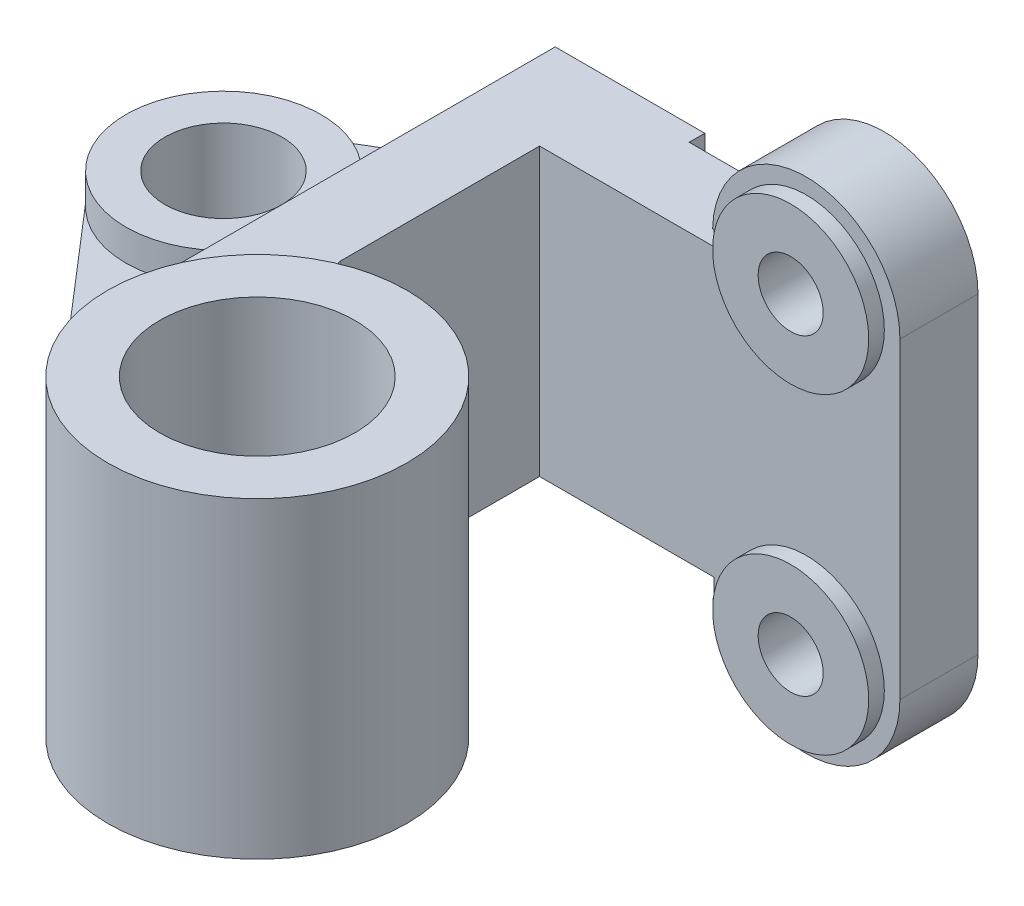
ISO-10303-21;
HEADER;
FILE_DESCRIPTION(('STEP AP214'),'2;1');
FILE_NAME('part.step','',(''),(''),'','','');
FILE_SCHEMA(('AUTOMOTIVE_DESIGN { 1 0 10303 214 1 1 1 1 }'));
ENDSEC;
DATA;
#1=APPLICATION_CONTEXT('core data for automotive mechanical design processes');
#2=APPLICATION_PROTOCOL_DEFINITION('international standard','automotive_design',2000,#1);
#3=PRODUCT_CONTEXT('',#1,'mechanical');
#4=PRODUCT('Part','Part','',(#3));
#5=PRODUCT_RELATED_PRODUCT_CATEGORY('part','',(#4));
#6=PRODUCT_DEFINITION_FORMATION('','',#4);
#7=PRODUCT_DEFINITION_CONTEXT('part definition',#1,'design');
#8=PRODUCT_DEFINITION('design','',#6,#7);
#9=PRODUCT_DEFINITION_SHAPE('','',#8);
#10=(LENGTH_UNIT() NAMED_UNIT(*) SI_UNIT(.MILLI.,.METRE.));
#11=(NAMED_UNIT(*) PLANE_ANGLE_UNIT() SI_UNIT($,.RADIAN.));
#12=(NAMED_UNIT(*) SI_UNIT($,.STERADIAN.) SOLID_ANGLE_UNIT());
#13=UNCERTAINTY_MEASURE_WITH_UNIT(LENGTH_MEASURE(1.E-05),#10,'distance_accuracy_value','');
#14=(GEOMETRIC_REPRESENTATION_CONTEXT(3) GLOBAL_UNCERTAINTY_ASSIGNED_CONTEXT((#13)) GLOBAL_UNIT_ASSIGNED_CONTEXT((#10,
#11,#12)) REPRESENTATION_CONTEXT('',''));
#15=CARTESIAN_POINT('',(0.,0.,0.));
#16=DIRECTION('',(0.,0.,1.));
#17=DIRECTION('',(1.,0.,0.));
#18=AXIS2_PLACEMENT_3D('',#15,#16,#17);
#19=CARTESIAN_POINT('',(-132.5,55.,151.));
#20=DIRECTION('',(1.,0.,0.));
#21=DIRECTION('',(0.,0.,-1.));
#22=AXIS2_PLACEMENT_3D('',#19,#20,#21);
#23=PLANE('',#22);
#24=DIRECTION('',(0.,0.,1.));
#25=VECTOR('',#24,1.);
#26=CARTESIAN_POINT('',(-132.5,-13.,151.));
#27=LINE('',#26,#25);
#28=CARTESIAN_POINT('',(-132.5,-13.,-21.));
#29=VERTEX_POINT('',#28);
#30=CARTESIAN_POINT('',(-132.5,-13.,151.));
#31=VERTEX_POINT('',#30);
#32=EDGE_CURVE('E59',#29,#31,#27,.T.);
#33=ORIENTED_EDGE('',*,*,#32,.F.);
#34=DIRECTION('',(0.,-1.,0.));
#35=VECTOR('',#34,1.);
#36=CARTESIAN_POINT('',(-132.5,55.,-21.));
#37=LINE('',#36,#35);
#38=CARTESIAN_POINT('',(-132.5,-55.,-21.));
#39=VERTEX_POINT('',#38);
#40=EDGE_CURVE('E314',#29,#39,#37,.T.);
#41=ORIENTED_EDGE('',*,*,#40,.T.);
#42=DIRECTION('',(0.,0.,1.));
#43=VECTOR('',#42,1.);
#44=CARTESIAN_POINT('',(-132.5,-55.,151.));
#45=LINE('',#44,#43);
#46=CARTESIAN_POINT('',(-132.5,-55.,151.));
#47=VERTEX_POINT('',#46);
#48=EDGE_CURVE('E283',#39,#47,#45,.T.);
#49=ORIENTED_EDGE('',*,*,#48,.T.);
#50=DIRECTION('',(0.,-1.,0.));
#51=VECTOR('',#50,1.);
#52=CARTESIAN_POINT('',(-132.5,55.,151.));
#53=LINE('',#52,#51);
#54=EDGE_CURVE('E298',#31,#47,#53,.T.);
#55=ORIENTED_EDGE('',*,*,#54,.F.);
#56=EDGE_LOOP('',(#33,#41,#49,#55));
#57=FACE_BOUND('',#56,.T.);
#58=ADVANCED_FACE('F43',(#57),#23,.F.);
#59=CARTESIAN_POINT('',(0.,60.,15.));
#60=DIRECTION('',(0.,0.,1.));
#61=DIRECTION('',(1.,0.,0.));
#62=AXIS2_PLACEMENT_3D('',#59,#60,#61);
#63=PLANE('',#62);
#64=DIRECTION('',(-1.,0.,0.));
#65=VECTOR('',#64,1.);
#66=CARTESIAN_POINT('',(0.,-55.,15.));
#67=LINE('',#66,#65);
#68=CARTESIAN_POINT('',(-35.5,-55.,15.));
#69=VERTEX_POINT('',#68);
#70=CARTESIAN_POINT('',(-102.5,-55.,15.));
#71=VERTEX_POINT('',#70);
#72=EDGE_CURVE('E248',#69,#71,#67,.T.);
#73=ORIENTED_EDGE('',*,*,#72,.F.);
#74=DIRECTION('',(0.,-1.,0.));
#75=VECTOR('',#74,1.);
#76=CARTESIAN_POINT('',(-35.5,60.,15.));
#77=LINE('',#76,#75);
#78=CARTESIAN_POINT('',(-35.5,-62.1816735998895,15.));
#79=VERTEX_POINT('',#78);
#80=EDGE_CURVE('E263',#69,#79,#77,.T.);
#81=ORIENTED_EDGE('',*,*,#80,.T.);
#82=DIRECTION('',(1.,0.,0.));
#83=VECTOR('',#82,1.);
#84=CARTESIAN_POINT('',(0.,-62.1816735998895,15.));
#85=LINE('',#84,#83);
#86=CARTESIAN_POINT('',(-35.9338322518423,-62.1816735998895,15.));
#87=VERTEX_POINT('',#86);
#88=EDGE_CURVE('E253',#87,#79,#85,.T.);
#89=ORIENTED_EDGE('',*,*,#88,.F.);
#90=CARTESIAN_POINT('',(0.,-60.,15.));
#91=DIRECTION('',(0.,0.,1.));
#92=DIRECTION('',(1.,0.,0.));
#93=AXIS2_PLACEMENT_3D('',#90,#91,#92);
#94=CIRCLE('',#93,36.);
#95=CARTESIAN_POINT('',(36.,-60.,15.));
#96=VERTEX_POINT('',#95);
#97=EDGE_CURVE('E364',#87,#96,#94,.T.);
#98=ORIENTED_EDGE('',*,*,#97,.T.);
#99=DIRECTION('',(0.,1.,0.));
#100=VECTOR('',#99,1.);
#101=CARTESIAN_POINT('',(36.,60.,15.));
#102=LINE('',#101,#100);
#103=CARTESIAN_POINT('',(36.,60.,15.));
#104=VERTEX_POINT('',#103);
#105=EDGE_CURVE('E370',#96,#104,#102,.T.);
#106=ORIENTED_EDGE('',*,*,#105,.T.);
#107=CARTESIAN_POINT('',(0.,60.,15.));
#108=DIRECTION('',(0.,0.,1.));
#109=DIRECTION('',(1.,0.,0.));
#110=AXIS2_PLACEMENT_3D('',#107,#108,#109);
#111=CIRCLE('',#110,36.);
#112=CARTESIAN_POINT('',(-35.9930063884241,60.7095710837273,15.));
#113=VERTEX_POINT('',#112);
#114=EDGE_CURVE('E363',#104,#113,#111,.T.);
#115=ORIENTED_EDGE('',*,*,#114,.T.);
#116=DIRECTION('',(-1.,0.,0.));
#117=VECTOR('',#116,1.);
#118=CARTESIAN_POINT('',(0.,60.7095710837273,15.));
#119=LINE('',#118,#117);
#120=CARTESIAN_POINT('',(-35.5,60.7095710837273,15.));
#121=VERTEX_POINT('',#120);
#122=EDGE_CURVE('E258',#121,#113,#119,.T.);
#123=ORIENTED_EDGE('',*,*,#122,.F.);
#124=DIRECTION('',(0.,1.,0.));
#125=VECTOR('',#124,1.);
#126=CARTESIAN_POINT('',(-35.5,60.,15.));
#127=LINE('',#126,#125);
#128=CARTESIAN_POINT('',(-35.5,55.,15.));
#129=VERTEX_POINT('',#128);
#130=EDGE_CURVE('E262',#129,#121,#127,.T.);
#131=ORIENTED_EDGE('',*,*,#130,.F.);
#132=DIRECTION('',(1.,0.,0.));
#133=VECTOR('',#132,1.);
#134=CARTESIAN_POINT('',(0.,55.,15.));
#135=LINE('',#134,#133);
#136=CARTESIAN_POINT('',(-102.5,55.,15.));
#137=VERTEX_POINT('',#136);
#138=EDGE_CURVE('E244',#137,#129,#135,.T.);
#139=ORIENTED_EDGE('',*,*,#138,.F.);
#140=DIRECTION('',(0.,-1.,0.));
#141=VECTOR('',#140,1.);
#142=CARTESIAN_POINT('',(-102.5,55.,15.));
#143=LINE('',#142,#141);
#144=EDGE_CURVE('E321',#137,#71,#143,.T.);
#145=ORIENTED_EDGE('',*,*,#144,.T.);
#146=EDGE_LOOP('',(#73,#81,#89,#98,#106,#115,#123,#131,#139,#145));
#147=FACE_BOUND('',#146,.T.);
#148=CARTESIAN_POINT('',(0.,60.,15.));
#149=DIRECTION('',(0.,0.,1.));
#150=DIRECTION('',(1.,0.,0.));
#151=AXIS2_PLACEMENT_3D('',#148,#149,#150);
#152=CIRCLE('',#151,30.);
#153=CARTESIAN_POINT('',(30.,60.,15.));
#154=VERTEX_POINT('',#153);
#155=EDGE_CURVE('E338',#154,#154,#152,.T.);
#156=ORIENTED_EDGE('',*,*,#155,.F.);
#157=EDGE_LOOP('',(#156));
#158=FACE_BOUND('',#157,.T.);
#159=CARTESIAN_POINT('',(0.,-60.,15.));
#160=DIRECTION('',(0.,0.,1.));
#161=DIRECTION('',(1.,0.,0.));
#162=AXIS2_PLACEMENT_3D('',#159,#160,#161);
#163=CIRCLE('',#162,30.);
#164=CARTESIAN_POINT('',(30.,-60.,15.));
#165=VERTEX_POINT('',#164);
#166=EDGE_CURVE('E346',#165,#165,#163,.T.);
#167=ORIENTED_EDGE('',*,*,#166,.F.);
#168=EDGE_LOOP('',(#167));
#169=FACE_BOUND('',#168,.T.);
#170=ADVANCED_FACE('F430',(#147,#158,#169),#63,.T.);
#171=CARTESIAN_POINT('',(0.,60.,-15.));
#172=DIRECTION('',(0.,0.,1.));
#173=DIRECTION('',(1.,0.,0.));
#174=AXIS2_PLACEMENT_3D('',#171,#172,#173);
#175=PLANE('',#174);
#176=DIRECTION('',(0.,-1.,0.));
#177=VECTOR('',#176,1.);
#178=CARTESIAN_POINT('',(-35.5,60.,-15.));
#179=LINE('',#178,#177);
#180=CARTESIAN_POINT('',(-35.5,-55.,-15.));
#181=VERTEX_POINT('',#180);
#182=CARTESIAN_POINT('',(-35.5,-62.1816735998895,-15.));
#183=VERTEX_POINT('',#182);
#184=EDGE_CURVE('E386',#181,#183,#179,.T.);
#185=ORIENTED_EDGE('',*,*,#184,.F.);
#186=DIRECTION('',(-1.,0.,0.));
#187=VECTOR('',#186,1.);
#188=CARTESIAN_POINT('',(0.,-55.,-15.));
#189=LINE('',#188,#187);
#190=CARTESIAN_POINT('',(-75.,-55.,-15.));
#191=VERTEX_POINT('',#190);
#192=EDGE_CURVE('E250',#181,#191,#189,.T.);
#193=ORIENTED_EDGE('',*,*,#192,.T.);
#194=DIRECTION('',(0.,-1.,0.));
#195=VECTOR('',#194,1.);
#196=CARTESIAN_POINT('',(-75.,55.,-15.));
#197=LINE('',#196,#195);
#198=CARTESIAN_POINT('',(-75.,55.,-15.));
#199=VERTEX_POINT('',#198);
#200=EDGE_CURVE('E322',#199,#191,#197,.T.);
#201=ORIENTED_EDGE('',*,*,#200,.F.);
#202=DIRECTION('',(1.,0.,0.));
#203=VECTOR('',#202,1.);
#204=CARTESIAN_POINT('',(0.,55.,-15.));
#205=LINE('',#204,#203);
#206=CARTESIAN_POINT('',(-35.5,55.,-15.));
#207=VERTEX_POINT('',#206);
#208=EDGE_CURVE('E238',#199,#207,#205,.T.);
#209=ORIENTED_EDGE('',*,*,#208,.T.);
#210=DIRECTION('',(0.,1.,0.));
#211=VECTOR('',#210,1.);
#212=CARTESIAN_POINT('',(-35.5,60.,-15.));
#213=LINE('',#212,#211);
#214=CARTESIAN_POINT('',(-35.5,60.7095710837273,-15.));
#215=VERTEX_POINT('',#214);
#216=EDGE_CURVE('E387',#207,#215,#213,.T.);
#217=ORIENTED_EDGE('',*,*,#216,.T.);
#218=DIRECTION('',(-1.,0.,0.));
#219=VECTOR('',#218,1.);
#220=CARTESIAN_POINT('',(0.,60.7095710837273,-15.));
#221=LINE('',#220,#219);
#222=CARTESIAN_POINT('',(-35.9930063884241,60.7095710837273,-15.));
#223=VERTEX_POINT('',#222);
#224=EDGE_CURVE('E260',#215,#223,#221,.T.);
#225=ORIENTED_EDGE('',*,*,#224,.T.);
#226=CARTESIAN_POINT('',(0.,60.,-15.));
#227=DIRECTION('',(0.,0.,1.));
#228=DIRECTION('',(1.,0.,0.));
#229=AXIS2_PLACEMENT_3D('',#226,#227,#228);
#230=CIRCLE('',#229,36.);
#231=CARTESIAN_POINT('',(36.,60.,-15.));
#232=VERTEX_POINT('',#231);
#233=EDGE_CURVE('E359',#232,#223,#230,.T.);
#234=ORIENTED_EDGE('',*,*,#233,.F.);
#235=DIRECTION('',(0.,1.,0.));
#236=VECTOR('',#235,1.);
#237=CARTESIAN_POINT('',(36.,60.,-15.));
#238=LINE('',#237,#236);
#239=CARTESIAN_POINT('',(36.,-60.,-15.));
#240=VERTEX_POINT('',#239);
#241=EDGE_CURVE('E362',#240,#232,#238,.T.);
#242=ORIENTED_EDGE('',*,*,#241,.F.);
#243=CARTESIAN_POINT('',(0.,-60.,-15.));
#244=DIRECTION('',(0.,0.,1.));
#245=DIRECTION('',(1.,0.,0.));
#246=AXIS2_PLACEMENT_3D('',#243,#244,#245);
#247=CIRCLE('',#246,36.);
#248=CARTESIAN_POINT('',(-35.9338322518424,-62.1816735998895,-15.));
#249=VERTEX_POINT('',#248);
#250=EDGE_CURVE('E375',#249,#240,#247,.T.);
#251=ORIENTED_EDGE('',*,*,#250,.F.);
#252=DIRECTION('',(1.,0.,0.));
#253=VECTOR('',#252,1.);
#254=CARTESIAN_POINT('',(0.,-62.1816735998895,-15.));
#255=LINE('',#254,#253);
#256=EDGE_CURVE('E255',#249,#183,#255,.T.);
#257=ORIENTED_EDGE('',*,*,#256,.T.);
#258=EDGE_LOOP('',(#185,#193,#201,#209,#217,#225,#234,#242,#251,#257));
#259=FACE_BOUND('',#258,.T.);
#260=CARTESIAN_POINT('',(0.,60.,-15.));
#261=DIRECTION('',(0.,0.,1.));
#262=DIRECTION('',(1.,0.,0.));
#263=AXIS2_PLACEMENT_3D('',#260,#261,#262);
#264=CIRCLE('',#263,12.5);
#265=CARTESIAN_POINT('',(12.5,60.,-15.));
#266=VERTEX_POINT('',#265);
#267=EDGE_CURVE('E357',#266,#266,#264,.T.);
#268=ORIENTED_EDGE('',*,*,#267,.T.);
#269=EDGE_LOOP('',(#268));
#270=FACE_BOUND('',#269,.T.);
#271=CARTESIAN_POINT('',(0.,-60.,-15.));
#272=DIRECTION('',(0.,0.,1.));
#273=DIRECTION('',(1.,0.,0.));
#274=AXIS2_PLACEMENT_3D('',#271,#272,#273);
#275=CIRCLE('',#274,12.5);
#276=CARTESIAN_POINT('',(12.5,-60.,-15.));
#277=VERTEX_POINT('',#276);
#278=EDGE_CURVE('E355',#277,#277,#275,.T.);
#279=ORIENTED_EDGE('',*,*,#278,.T.);
#280=EDGE_LOOP('',(#279));
#281=FACE_BOUND('',#280,.T.);
#282=ADVANCED_FACE('F434',(#259,#270,#281),#175,.F.);
#283=CARTESIAN_POINT('',(0.,60.,15.));
#284=DIRECTION('',(0.,0.,-1.));
#285=DIRECTION('',(-1.,0.,0.));
#286=AXIS2_PLACEMENT_3D('',#283,#284,#285);
#287=CYLINDRICAL_SURFACE('',#286,36.);
#288=ORIENTED_EDGE('',*,*,#233,.T.);
#289=DIRECTION('',(0.,0.,-1.));
#290=VECTOR('',#289,1.);
#291=CARTESIAN_POINT('',(-35.9930063884241,60.7095710837273,15.));
#292=LINE('',#291,#290);
#293=EDGE_CURVE('E384',#223,#113,#292,.F.);
#294=ORIENTED_EDGE('',*,*,#293,.T.);
#295=ORIENTED_EDGE('',*,*,#114,.F.);
#296=DIRECTION('',(0.,0.,-1.));
#297=VECTOR('',#296,1.);
#298=CARTESIAN_POINT('',(36.,60.,15.));
#299=LINE('',#298,#297);
#300=EDGE_CURVE('E367',#104,#232,#299,.T.);
#301=ORIENTED_EDGE('',*,*,#300,.T.);
#302=EDGE_LOOP('',(#288,#294,#295,#301));
#303=FACE_BOUND('',#302,.T.);
#304=ADVANCED_FACE('F44',(#303),#287,.T.);
#305=CARTESIAN_POINT('',(0.,-60.,15.));
#306=DIRECTION('',(0.,0.,-1.));
#307=DIRECTION('',(-1.,0.,0.));
#308=AXIS2_PLACEMENT_3D('',#305,#306,#307);
#309=CYLINDRICAL_SURFACE('',#308,36.);
#310=ORIENTED_EDGE('',*,*,#97,.F.);
#311=DIRECTION('',(0.,0.,-1.));
#312=VECTOR('',#311,1.);
#313=CARTESIAN_POINT('',(-35.9338322518423,-62.1816735998895,15.));
#314=LINE('',#313,#312);
#315=EDGE_CURVE('E379',#87,#249,#314,.T.);
#316=ORIENTED_EDGE('',*,*,#315,.T.);
#317=ORIENTED_EDGE('',*,*,#250,.T.);
#318=DIRECTION('',(0.,0.,-1.));
#319=VECTOR('',#318,1.);
#320=CARTESIAN_POINT('',(36.,-60.,15.));
#321=LINE('',#320,#319);
#322=EDGE_CURVE('E380',#96,#240,#321,.T.);
#323=ORIENTED_EDGE('',*,*,#322,.F.);
#324=EDGE_LOOP('',(#310,#316,#317,#323));
#325=FACE_BOUND('',#324,.T.);
#326=ADVANCED_FACE('F505',(#325),#309,.T.);
#327=CARTESIAN_POINT('',(36.,60.,15.));
#328=DIRECTION('',(-1.,0.,0.));
#329=DIRECTION('',(0.,-1.,0.));
#330=AXIS2_PLACEMENT_3D('',#327,#328,#329);
#331=PLANE('',#330);
#332=ORIENTED_EDGE('',*,*,#241,.T.);
#333=ORIENTED_EDGE('',*,*,#300,.F.);
#334=ORIENTED_EDGE('',*,*,#105,.F.);
#335=ORIENTED_EDGE('',*,*,#322,.T.);
#336=EDGE_LOOP('',(#332,#333,#334,#335));
#337=FACE_BOUND('',#336,.T.);
#338=ADVANCED_FACE('F510',(#337),#331,.F.);
#339=CARTESIAN_POINT('',(0.,60.,15.));
#340=DIRECTION('',(0.,0.,-1.));
#341=DIRECTION('',(-1.,0.,0.));
#342=AXIS2_PLACEMENT_3D('',#339,#340,#341);
#343=CYLINDRICAL_SURFACE('',#342,12.5);
#344=ORIENTED_EDGE('',*,*,#267,.F.);
#345=EDGE_LOOP('',(#344));
#346=FACE_BOUND('',#345,.T.);
#347=CARTESIAN_POINT('',(0.,60.,21.));
#348=DIRECTION('',(0.,0.,-1.));
#349=DIRECTION('',(-1.,0.,0.));
#350=AXIS2_PLACEMENT_3D('',#347,#348,#349);
#351=CIRCLE('',#350,12.5);
#352=CARTESIAN_POINT('',(-12.5,60.,21.));
#353=VERTEX_POINT('',#352);
#354=EDGE_CURVE('E337',#353,#353,#351,.T.);
#355=ORIENTED_EDGE('',*,*,#354,.F.);
#356=EDGE_LOOP('',(#355));
#357=FACE_BOUND('',#356,.T.);
#358=ADVANCED_FACE('F562',(#346,#357),#343,.F.);
#359=CARTESIAN_POINT('',(0.,-60.,15.));
#360=DIRECTION('',(0.,0.,-1.));
#361=DIRECTION('',(-1.,0.,0.));
#362=AXIS2_PLACEMENT_3D('',#359,#360,#361);
#363=CYLINDRICAL_SURFACE('',#362,12.5);
#364=ORIENTED_EDGE('',*,*,#278,.F.);
#365=EDGE_LOOP('',(#364));
#366=FACE_BOUND('',#365,.T.);
#367=CARTESIAN_POINT('',(0.,-60.,21.));
#368=DIRECTION('',(0.,0.,-1.));
#369=DIRECTION('',(-1.,0.,0.));
#370=AXIS2_PLACEMENT_3D('',#367,#368,#369);
#371=CIRCLE('',#370,12.5);
#372=CARTESIAN_POINT('',(-12.5,-60.,21.));
#373=VERTEX_POINT('',#372);
#374=EDGE_CURVE('E340',#373,#373,#371,.T.);
#375=ORIENTED_EDGE('',*,*,#374,.F.);
#376=EDGE_LOOP('',(#375));
#377=FACE_BOUND('',#376,.T.);
#378=ADVANCED_FACE('F557',(#366,#377),#363,.F.);
#379=CARTESIAN_POINT('',(0.,-60.,21.));
#380=DIRECTION('',(0.,0.,-1.));
#381=DIRECTION('',(-1.,0.,0.));
#382=AXIS2_PLACEMENT_3D('',#379,#380,#381);
#383=CYLINDRICAL_SURFACE('',#382,30.);
#384=CARTESIAN_POINT('',(0.,-60.,21.));
#385=DIRECTION('',(0.,0.,1.));
#386=DIRECTION('',(1.,0.,0.));
#387=AXIS2_PLACEMENT_3D('',#384,#385,#386);
#388=CIRCLE('',#387,30.);
#389=CARTESIAN_POINT('',(30.,-60.,21.));
#390=VERTEX_POINT('',#389);
#391=EDGE_CURVE('E348',#390,#390,#388,.T.);
#392=ORIENTED_EDGE('',*,*,#391,.F.);
#393=EDGE_LOOP('',(#392));
#394=FACE_BOUND('',#393,.T.);
#395=ORIENTED_EDGE('',*,*,#166,.T.);
#396=EDGE_LOOP('',(#395));
#397=FACE_BOUND('',#396,.T.);
#398=ADVANCED_FACE('F558',(#394,#397),#383,.T.);
#399=CARTESIAN_POINT('',(0.,-60.,21.));
#400=DIRECTION('',(0.,0.,1.));
#401=DIRECTION('',(1.,0.,0.));
#402=AXIS2_PLACEMENT_3D('',#399,#400,#401);
#403=PLANE('',#402);
#404=ORIENTED_EDGE('',*,*,#374,.T.);
#405=EDGE_LOOP('',(#404));
#406=FACE_BOUND('',#405,.T.);
#407=ORIENTED_EDGE('',*,*,#391,.T.);
#408=EDGE_LOOP('',(#407));
#409=FACE_BOUND('',#408,.T.);
#410=ADVANCED_FACE('F552',(#406,#409),#403,.T.);
#411=CARTESIAN_POINT('',(0.,60.,21.));
#412=DIRECTION('',(0.,0.,-1.));
#413=DIRECTION('',(-1.,0.,0.));
#414=AXIS2_PLACEMENT_3D('',#411,#412,#413);
#415=CYLINDRICAL_SURFACE('',#414,30.);
#416=CARTESIAN_POINT('',(0.,60.,21.));
#417=DIRECTION('',(0.,0.,1.));
#418=DIRECTION('',(1.,0.,0.));
#419=AXIS2_PLACEMENT_3D('',#416,#417,#418);
#420=CIRCLE('',#419,30.);
#421=CARTESIAN_POINT('',(30.,60.,21.));
#422=VERTEX_POINT('',#421);
#423=EDGE_CURVE('E344',#422,#422,#420,.T.);
#424=ORIENTED_EDGE('',*,*,#423,.F.);
#425=EDGE_LOOP('',(#424));
#426=FACE_BOUND('',#425,.T.);
#427=ORIENTED_EDGE('',*,*,#155,.T.);
#428=EDGE_LOOP('',(#427));
#429=FACE_BOUND('',#428,.T.);
#430=ADVANCED_FACE('F548',(#426,#429),#415,.T.);
#431=CARTESIAN_POINT('',(0.,60.,21.));
#432=DIRECTION('',(0.,0.,1.));
#433=DIRECTION('',(1.,0.,0.));
#434=AXIS2_PLACEMENT_3D('',#431,#432,#433);
#435=PLANE('',#434);
#436=ORIENTED_EDGE('',*,*,#354,.T.);
#437=EDGE_LOOP('',(#436));
#438=FACE_BOUND('',#437,.T.);
#439=ORIENTED_EDGE('',*,*,#423,.T.);
#440=EDGE_LOOP('',(#439));
#441=FACE_BOUND('',#440,.T.);
#442=ADVANCED_FACE('F531',(#438,#441),#435,.T.);
#443=CARTESIAN_POINT('',(-75.,55.,151.));
#444=DIRECTION('',(0.,1.,0.));
#445=DIRECTION('',(0.,0.,1.));
#446=AXIS2_PLACEMENT_3D('',#443,#444,#445);
#447=PLANE('',#446);
#448=DIRECTION('',(0.,0.,-1.));
#449=VECTOR('',#448,1.);
#450=CARTESIAN_POINT('',(-102.5,55.,15.));
#451=LINE('',#450,#449);
#452=CARTESIAN_POINT('',(-102.5,55.,91.5));
#453=VERTEX_POINT('',#452);
#454=EDGE_CURVE('E288',#453,#137,#451,.T.);
#455=ORIENTED_EDGE('',*,*,#454,.T.);
#456=ORIENTED_EDGE('',*,*,#138,.T.);
#457=DIRECTION('',(0.,0.,1.));
#458=VECTOR('',#457,1.);
#459=CARTESIAN_POINT('',(-35.5,55.,-21.));
#460=LINE('',#459,#458);
#461=EDGE_CURVE('E229',#207,#129,#460,.T.);
#462=ORIENTED_EDGE('',*,*,#461,.F.);
#463=ORIENTED_EDGE('',*,*,#208,.F.);
#464=DIRECTION('',(0.,0.,-1.));
#465=VECTOR('',#464,1.);
#466=CARTESIAN_POINT('',(-75.,55.,-21.));
#467=LINE('',#466,#465);
#468=CARTESIAN_POINT('',(-75.,55.,-21.));
#469=VERTEX_POINT('',#468);
#470=EDGE_CURVE('E286',#199,#469,#467,.T.);
#471=ORIENTED_EDGE('',*,*,#470,.T.);
#472=DIRECTION('',(-1.,0.,0.));
#473=VECTOR('',#472,1.);
#474=CARTESIAN_POINT('',(-132.5,55.,-21.));
#475=LINE('',#474,#473);
#476=CARTESIAN_POINT('',(-132.5,55.,-21.));
#477=VERTEX_POINT('',#476);
#478=EDGE_CURVE('E292',#469,#477,#475,.T.);
#479=ORIENTED_EDGE('',*,*,#478,.T.);
#480=DIRECTION('',(0.,0.,1.));
#481=VECTOR('',#480,1.);
#482=CARTESIAN_POINT('',(-132.5,55.,151.));
#483=LINE('',#482,#481);
#484=CARTESIAN_POINT('',(-132.5,55.,151.));
#485=VERTEX_POINT('',#484);
#486=EDGE_CURVE('E295',#477,#485,#483,.T.);
#487=ORIENTED_EDGE('',*,*,#486,.T.);
#488=CARTESIAN_POINT('',(-75.,55.,151.));
#489=DIRECTION('',(0.,-1.,0.));
#490=DIRECTION('',(0.,0.,1.));
#491=AXIS2_PLACEMENT_3D('',#488,#489,#490);
#492=CIRCLE('',#491,57.5);
#493=CARTESIAN_POINT('',(-75.,55.,93.5));
#494=VERTEX_POINT('',#493);
#495=EDGE_CURVE('E278',#485,#494,#492,.T.);
#496=ORIENTED_EDGE('',*,*,#495,.T.);
#497=DIRECTION('',(-1.,0.,0.));
#498=VECTOR('',#497,1.);
#499=CARTESIAN_POINT('',(-100.5,55.,93.5));
#500=LINE('',#499,#498);
#501=CARTESIAN_POINT('',(-100.5,55.,93.5));
#502=VERTEX_POINT('',#501);
#503=EDGE_CURVE('E284',#494,#502,#500,.T.);
#504=ORIENTED_EDGE('',*,*,#503,.T.);
#505=CARTESIAN_POINT('',(-100.5,55.,91.5));
#506=DIRECTION('',(0.,-1.,0.));
#507=DIRECTION('',(0.,0.,1.));
#508=AXIS2_PLACEMENT_3D('',#505,#506,#507);
#509=CIRCLE('',#508,2.);
#510=EDGE_CURVE('E287',#502,#453,#509,.T.);
#511=ORIENTED_EDGE('',*,*,#510,.T.);
#512=EDGE_LOOP('',(#455,#456,#462,#463,#471,#479,#487,#496,#504,#511));
#513=FACE_BOUND('',#512,.T.);
#514=ADVANCED_FACE('F453',(#513),#447,.T.);
#515=CARTESIAN_POINT('',(-75.,-55.,151.));
#516=DIRECTION('',(0.,1.,0.));
#517=DIRECTION('',(0.,0.,1.));
#518=AXIS2_PLACEMENT_3D('',#515,#516,#517);
#519=PLANE('',#518);
#520=ORIENTED_EDGE('',*,*,#72,.T.);
#521=DIRECTION('',(0.,0.,-1.));
#522=VECTOR('',#521,1.);
#523=CARTESIAN_POINT('',(-102.5,-55.,15.));
#524=LINE('',#523,#522);
#525=CARTESIAN_POINT('',(-102.5,-55.,91.5));
#526=VERTEX_POINT('',#525);
#527=EDGE_CURVE('E303',#526,#71,#524,.T.);
#528=ORIENTED_EDGE('',*,*,#527,.F.);
#529=CARTESIAN_POINT('',(-100.5,-55.,91.5));
#530=DIRECTION('',(0.,-1.,0.));
#531=DIRECTION('',(0.,0.,1.));
#532=AXIS2_PLACEMENT_3D('',#529,#530,#531);
#533=CIRCLE('',#532,2.);
#534=CARTESIAN_POINT('',(-100.5,-55.,93.5));
#535=VERTEX_POINT('',#534);
#536=EDGE_CURVE('E301',#535,#526,#533,.T.);
#537=ORIENTED_EDGE('',*,*,#536,.F.);
#538=DIRECTION('',(-1.,0.,0.));
#539=VECTOR('',#538,1.);
#540=CARTESIAN_POINT('',(-100.5,-55.,93.5));
#541=LINE('',#540,#539);
#542=CARTESIAN_POINT('',(-75.,-55.,93.5));
#543=VERTEX_POINT('',#542);
#544=EDGE_CURVE('E299',#543,#535,#541,.T.);
#545=ORIENTED_EDGE('',*,*,#544,.F.);
#546=CARTESIAN_POINT('',(-75.,-55.,151.));
#547=DIRECTION('',(0.,-1.,0.));
#548=DIRECTION('',(0.,0.,1.));
#549=AXIS2_PLACEMENT_3D('',#546,#547,#548);
#550=CIRCLE('',#549,57.5);
#551=EDGE_CURVE('E280',#47,#543,#550,.T.);
#552=ORIENTED_EDGE('',*,*,#551,.F.);
#553=ORIENTED_EDGE('',*,*,#48,.F.);
#554=DIRECTION('',(-1.,0.,0.));
#555=VECTOR('',#554,1.);
#556=CARTESIAN_POINT('',(-132.5,-55.,-21.));
#557=LINE('',#556,#555);
#558=CARTESIAN_POINT('',(-75.,-55.,-21.));
#559=VERTEX_POINT('',#558);
#560=EDGE_CURVE('E310',#559,#39,#557,.T.);
#561=ORIENTED_EDGE('',*,*,#560,.F.);
#562=DIRECTION('',(0.,0.,-1.));
#563=VECTOR('',#562,1.);
#564=CARTESIAN_POINT('',(-75.,-55.,-21.));
#565=LINE('',#564,#563);
#566=EDGE_CURVE('E304',#191,#559,#565,.T.);
#567=ORIENTED_EDGE('',*,*,#566,.F.);
#568=ORIENTED_EDGE('',*,*,#192,.F.);
#569=DIRECTION('',(0.,0.,-1.));
#570=VECTOR('',#569,1.);
#571=CARTESIAN_POINT('',(-35.5,-55.,-21.));
#572=LINE('',#571,#570);
#573=EDGE_CURVE('E234',#69,#181,#572,.T.);
#574=ORIENTED_EDGE('',*,*,#573,.F.);
#575=EDGE_LOOP('',(#520,#528,#537,#545,#552,#553,#561,#567,#568,#574));
#576=FACE_BOUND('',#575,.T.);
#577=ADVANCED_FACE('F465',(#576),#519,.F.);
#578=CARTESIAN_POINT('',(-100.5,55.,93.5));
#579=DIRECTION('',(0.,0.,1.));
#580=DIRECTION('',(1.,0.,0.));
#581=AXIS2_PLACEMENT_3D('',#578,#579,#580);
#582=PLANE('',#581);
#583=ORIENTED_EDGE('',*,*,#544,.T.);
#584=DIRECTION('',(0.,-1.,0.));
#585=VECTOR('',#584,1.);
#586=CARTESIAN_POINT('',(-100.5,55.,93.5));
#587=LINE('',#586,#585);
#588=EDGE_CURVE('E330',#502,#535,#587,.T.);
#589=ORIENTED_EDGE('',*,*,#588,.F.);
#590=ORIENTED_EDGE('',*,*,#503,.F.);
#591=DIRECTION('',(0.,-1.,0.));
#592=VECTOR('',#591,1.);
#593=CARTESIAN_POINT('',(-75.,55.,93.5));
#594=LINE('',#593,#592);
#595=EDGE_CURVE('E333',#494,#543,#594,.T.);
#596=ORIENTED_EDGE('',*,*,#595,.T.);
#597=EDGE_LOOP('',(#583,#589,#590,#596));
#598=FACE_BOUND('',#597,.T.);
#599=ADVANCED_FACE('F469',(#598),#582,.F.);
#600=CARTESIAN_POINT('',(-100.5,55.,91.5));
#601=DIRECTION('',(0.,-1.,0.));
#602=DIRECTION('',(0.,0.,-1.));
#603=AXIS2_PLACEMENT_3D('',#600,#601,#602);
#604=CYLINDRICAL_SURFACE('',#603,2.);
#605=ORIENTED_EDGE('',*,*,#536,.T.);
#606=DIRECTION('',(0.,-1.,0.));
#607=VECTOR('',#606,1.);
#608=CARTESIAN_POINT('',(-102.5,55.,91.5));
#609=LINE('',#608,#607);
#610=EDGE_CURVE('E327',#453,#526,#609,.T.);
#611=ORIENTED_EDGE('',*,*,#610,.F.);
#612=ORIENTED_EDGE('',*,*,#510,.F.);
#613=ORIENTED_EDGE('',*,*,#588,.T.);
#614=EDGE_LOOP('',(#605,#611,#612,#613));
#615=FACE_BOUND('',#614,.T.);
#616=ADVANCED_FACE('F476',(#615),#604,.F.);
#617=CARTESIAN_POINT('',(-102.5,55.,15.));
#618=DIRECTION('',(-1.,0.,0.));
#619=DIRECTION('',(0.,0.,1.));
#620=AXIS2_PLACEMENT_3D('',#617,#618,#619);
#621=PLANE('',#620);
#622=ORIENTED_EDGE('',*,*,#527,.T.);
#623=ORIENTED_EDGE('',*,*,#144,.F.);
#624=ORIENTED_EDGE('',*,*,#454,.F.);
#625=ORIENTED_EDGE('',*,*,#610,.T.);
#626=EDGE_LOOP('',(#622,#623,#624,#625));
#627=FACE_BOUND('',#626,.T.);
#628=ADVANCED_FACE('F480',(#627),#621,.F.);
#629=CARTESIAN_POINT('',(-75.,55.,-21.));
#630=DIRECTION('',(-1.,0.,0.));
#631=DIRECTION('',(0.,0.,1.));
#632=AXIS2_PLACEMENT_3D('',#629,#630,#631);
#633=PLANE('',#632);
#634=ORIENTED_EDGE('',*,*,#566,.T.);
#635=DIRECTION('',(0.,-1.,0.));
#636=VECTOR('',#635,1.);
#637=CARTESIAN_POINT('',(-75.,55.,-21.));
#638=LINE('',#637,#636);
#639=EDGE_CURVE('E319',#469,#559,#638,.T.);
#640=ORIENTED_EDGE('',*,*,#639,.F.);
#641=ORIENTED_EDGE('',*,*,#470,.F.);
#642=ORIENTED_EDGE('',*,*,#200,.T.);
#643=EDGE_LOOP('',(#634,#640,#641,#642));
#644=FACE_BOUND('',#643,.T.);
#645=ADVANCED_FACE('F446',(#644),#633,.F.);
#646=CARTESIAN_POINT('',(-132.5,55.,-21.));
#647=DIRECTION('',(0.,0.,1.));
#648=DIRECTION('',(1.,0.,0.));
#649=AXIS2_PLACEMENT_3D('',#646,#647,#648);
#650=PLANE('',#649);
#651=DIRECTION('',(0.,-1.,0.));
#652=VECTOR('',#651,1.);
#653=CARTESIAN_POINT('',(-132.5,13.,-21.));
#654=LINE('',#653,#652);
#655=CARTESIAN_POINT('',(-132.5,13.,-21.));
#656=VERTEX_POINT('',#655);
#657=EDGE_CURVE('E63',#656,#29,#654,.T.);
#658=ORIENTED_EDGE('',*,*,#657,.F.);
#659=EDGE_CURVE('E317',#477,#656,#37,.T.);
#660=ORIENTED_EDGE('',*,*,#659,.F.);
#661=ORIENTED_EDGE('',*,*,#478,.F.);
#662=ORIENTED_EDGE('',*,*,#639,.T.);
#663=ORIENTED_EDGE('',*,*,#560,.T.);
#664=ORIENTED_EDGE('',*,*,#40,.F.);
#665=EDGE_LOOP('',(#658,#660,#661,#662,#663,#664));
#666=FACE_BOUND('',#665,.T.);
#667=ADVANCED_FACE('F441',(#666),#650,.F.);
#668=ORIENTED_EDGE('',*,*,#659,.T.);
#669=DIRECTION('',(0.,0.,1.));
#670=VECTOR('',#669,1.);
#671=CARTESIAN_POINT('',(-132.5,13.,151.));
#672=LINE('',#671,#670);
#673=CARTESIAN_POINT('',(-132.5,13.,151.));
#674=VERTEX_POINT('',#673);
#675=EDGE_CURVE('E226',#656,#674,#672,.T.);
#676=ORIENTED_EDGE('',*,*,#675,.T.);
#677=EDGE_CURVE('E315',#485,#674,#53,.T.);
#678=ORIENTED_EDGE('',*,*,#677,.F.);
#679=ORIENTED_EDGE('',*,*,#486,.F.);
#680=EDGE_LOOP('',(#668,#676,#678,#679));
#681=FACE_BOUND('',#680,.T.);
#682=ADVANCED_FACE('F429',(#681),#23,.F.);
#683=CARTESIAN_POINT('',(-75.,60.,151.));
#684=DIRECTION('',(0.,-1.,0.));
#685=DIRECTION('',(0.,0.,-1.));
#686=AXIS2_PLACEMENT_3D('',#683,#684,#685);
#687=CYLINDRICAL_SURFACE('',#686,57.5);
#688=CARTESIAN_POINT('',(-75.,60.,151.));
#689=DIRECTION('',(0.,1.,0.));
#690=DIRECTION('',(0.,0.,1.));
#691=AXIS2_PLACEMENT_3D('',#688,#689,#690);
#692=CIRCLE('',#691,57.5);
#693=CARTESIAN_POINT('',(-75.,60.,208.5));
#694=VERTEX_POINT('',#693);
#695=EDGE_CURVE('E274',#694,#694,#692,.T.);
#696=ORIENTED_EDGE('',*,*,#695,.F.);
#697=EDGE_LOOP('',(#696));
#698=FACE_BOUND('',#697,.T.);
#699=CARTESIAN_POINT('',(-75.,-60.,151.));
#700=DIRECTION('',(0.,1.,0.));
#701=DIRECTION('',(0.,0.,1.));
#702=AXIS2_PLACEMENT_3D('',#699,#700,#701);
#703=CIRCLE('',#702,57.5);
#704=CARTESIAN_POINT('',(-75.,-60.,208.5));
#705=VERTEX_POINT('',#704);
#706=EDGE_CURVE('E272',#705,#705,#703,.T.);
#707=ORIENTED_EDGE('',*,*,#706,.T.);
#708=EDGE_LOOP('',(#707));
#709=FACE_BOUND('',#708,.T.);
#710=ORIENTED_EDGE('',*,*,#677,.T.);
#711=CARTESIAN_POINT('',(-75.,13.,151.));
#712=DIRECTION('',(0.,1.,0.));
#713=DIRECTION('',(0.,0.,1.));
#714=AXIS2_PLACEMENT_3D('',#711,#712,#713);
#715=CIRCLE('',#714,57.5);
#716=CARTESIAN_POINT('',(-118.556252792264,13.,188.538018630402));
#717=VERTEX_POINT('',#716);
#718=EDGE_CURVE('E51',#674,#717,#715,.T.);
#719=ORIENTED_EDGE('',*,*,#718,.T.);
#720=DIRECTION('',(0.,-1.,0.));
#721=VECTOR('',#720,1.);
#722=CARTESIAN_POINT('',(-118.556252792264,13.,188.538018630402));
#723=LINE('',#722,#721);
#724=CARTESIAN_POINT('',(-118.556252792264,-13.,188.538018630402));
#725=VERTEX_POINT('',#724);
#726=EDGE_CURVE('E210',#717,#725,#723,.T.);
#727=ORIENTED_EDGE('',*,*,#726,.T.);
#728=CARTESIAN_POINT('',(-75.,-13.,151.));
#729=DIRECTION('',(0.,1.,0.));
#730=DIRECTION('',(0.,0.,1.));
#731=AXIS2_PLACEMENT_3D('',#728,#729,#730);
#732=CIRCLE('',#731,57.5);
#733=EDGE_CURVE('E194',#31,#725,#732,.T.);
#734=ORIENTED_EDGE('',*,*,#733,.F.);
#735=ORIENTED_EDGE('',*,*,#54,.T.);
#736=ORIENTED_EDGE('',*,*,#551,.T.);
#737=ORIENTED_EDGE('',*,*,#595,.F.);
#738=ORIENTED_EDGE('',*,*,#495,.F.);
#739=EDGE_LOOP('',(#710,#719,#727,#734,#735,#736,#737,#738));
#740=FACE_BOUND('',#739,.T.);
#741=ADVANCED_FACE('F394',(#698,#709,#740),#687,.T.);
#742=CARTESIAN_POINT('',(-75.,60.,151.));
#743=DIRECTION('',(0.,1.,0.));
#744=DIRECTION('',(0.,0.,1.));
#745=AXIS2_PLACEMENT_3D('',#742,#743,#744);
#746=PLANE('',#745);
#747=ORIENTED_EDGE('',*,*,#695,.T.);
#748=EDGE_LOOP('',(#747));
#749=FACE_BOUND('',#748,.T.);
#750=CARTESIAN_POINT('',(-75.,60.,151.));
#751=DIRECTION('',(0.,1.,0.));
#752=DIRECTION('',(0.,0.,1.));
#753=AXIS2_PLACEMENT_3D('',#750,#751,#752);
#754=CIRCLE('',#753,37.5);
#755=CARTESIAN_POINT('',(-75.,60.,188.5));
#756=VERTEX_POINT('',#755);
#757=EDGE_CURVE('E268',#756,#756,#754,.T.);
#758=ORIENTED_EDGE('',*,*,#757,.F.);
#759=EDGE_LOOP('',(#758));
#760=FACE_BOUND('',#759,.T.);
#761=ADVANCED_FACE('F447',(#749,#760),#746,.T.);
#762=CARTESIAN_POINT('',(-75.,-60.,151.));
#763=DIRECTION('',(0.,1.,0.));
#764=DIRECTION('',(0.,0.,1.));
#765=AXIS2_PLACEMENT_3D('',#762,#763,#764);
#766=PLANE('',#765);
#767=ORIENTED_EDGE('',*,*,#706,.F.);
#768=EDGE_LOOP('',(#767));
#769=FACE_BOUND('',#768,.T.);
#770=CARTESIAN_POINT('',(-75.,-60.,151.));
#771=DIRECTION('',(0.,1.,0.));
#772=DIRECTION('',(0.,0.,1.));
#773=AXIS2_PLACEMENT_3D('',#770,#771,#772);
#774=CIRCLE('',#773,37.5);
#775=CARTESIAN_POINT('',(-75.,-60.,188.5));
#776=VERTEX_POINT('',#775);
#777=EDGE_CURVE('E270',#776,#776,#774,.T.);
#778=ORIENTED_EDGE('',*,*,#777,.T.);
#779=EDGE_LOOP('',(#778));
#780=FACE_BOUND('',#779,.T.);
#781=ADVANCED_FACE('F523',(#769,#780),#766,.F.);
#782=CARTESIAN_POINT('',(-75.,60.,151.));
#783=DIRECTION('',(0.,-1.,0.));
#784=DIRECTION('',(0.,0.,-1.));
#785=AXIS2_PLACEMENT_3D('',#782,#783,#784);
#786=CYLINDRICAL_SURFACE('',#785,37.5);
#787=ORIENTED_EDGE('',*,*,#757,.T.);
#788=EDGE_LOOP('',(#787));
#789=FACE_BOUND('',#788,.T.);
#790=ORIENTED_EDGE('',*,*,#777,.F.);
#791=EDGE_LOOP('',(#790));
#792=FACE_BOUND('',#791,.T.);
#793=ADVANCED_FACE('F521',(#789,#792),#786,.F.);
#794=CARTESIAN_POINT('',(-35.5,0.,0.));
#795=DIRECTION('',(-1.,0.,0.));
#796=DIRECTION('',(0.,0.,1.));
#797=AXIS2_PLACEMENT_3D('',#794,#795,#796);
#798=PLANE('',#797);
#799=ORIENTED_EDGE('',*,*,#573,.T.);
#800=ORIENTED_EDGE('',*,*,#184,.T.);
#801=DIRECTION('',(0.,0.,1.));
#802=VECTOR('',#801,1.);
#803=CARTESIAN_POINT('',(-35.5,-62.1816735998895,-21.));
#804=LINE('',#803,#802);
#805=EDGE_CURVE('E233',#183,#79,#804,.T.);
#806=ORIENTED_EDGE('',*,*,#805,.T.);
#807=ORIENTED_EDGE('',*,*,#80,.F.);
#808=EDGE_LOOP('',(#799,#800,#806,#807));
#809=FACE_BOUND('',#808,.T.);
#810=ADVANCED_FACE('F492',(#809),#798,.T.);
#811=CARTESIAN_POINT('',(-35.5,-62.1816735998895,-21.));
#812=DIRECTION('',(0.,-1.,0.));
#813=DIRECTION('',(0.,0.,-1.));
#814=AXIS2_PLACEMENT_3D('',#811,#812,#813);
#815=PLANE('',#814);
#816=ORIENTED_EDGE('',*,*,#88,.T.);
#817=ORIENTED_EDGE('',*,*,#805,.F.);
#818=ORIENTED_EDGE('',*,*,#256,.F.);
#819=ORIENTED_EDGE('',*,*,#315,.F.);
#820=EDGE_LOOP('',(#816,#817,#818,#819));
#821=FACE_BOUND('',#820,.T.);
#822=ADVANCED_FACE('F500',(#821),#815,.F.);
#823=CARTESIAN_POINT('',(-35.5,0.,0.));
#824=DIRECTION('',(1.,0.,0.));
#825=DIRECTION('',(0.,0.,-1.));
#826=AXIS2_PLACEMENT_3D('',#823,#824,#825);
#827=PLANE('',#826);
#828=ORIENTED_EDGE('',*,*,#130,.T.);
#829=DIRECTION('',(0.,0.,-1.));
#830=VECTOR('',#829,1.);
#831=CARTESIAN_POINT('',(-35.5,60.7095710837273,-21.));
#832=LINE('',#831,#830);
#833=EDGE_CURVE('E232',#121,#215,#832,.T.);
#834=ORIENTED_EDGE('',*,*,#833,.T.);
#835=ORIENTED_EDGE('',*,*,#216,.F.);
#836=ORIENTED_EDGE('',*,*,#461,.T.);
#837=EDGE_LOOP('',(#828,#834,#835,#836));
#838=FACE_BOUND('',#837,.T.);
#839=ADVANCED_FACE('F488',(#838),#827,.F.);
#840=CARTESIAN_POINT('',(-35.5,60.7095710837273,-21.));
#841=DIRECTION('',(0.,1.,0.));
#842=DIRECTION('',(0.,0.,1.));
#843=AXIS2_PLACEMENT_3D('',#840,#841,#842);
#844=PLANE('',#843);
#845=ORIENTED_EDGE('',*,*,#122,.T.);
#846=ORIENTED_EDGE('',*,*,#293,.F.);
#847=ORIENTED_EDGE('',*,*,#224,.F.);
#848=ORIENTED_EDGE('',*,*,#833,.F.);
#849=EDGE_LOOP('',(#845,#846,#847,#848));
#850=FACE_BOUND('',#849,.T.);
#851=ADVANCED_FACE('F512',(#850),#844,.F.);
#852=CARTESIAN_POINT('',(-44.0364383145327,13.,-73.7919440153795));
#853=DIRECTION('',(0.512451592326177,0.,0.858716114628324));
#854=DIRECTION('',(0.858716114628324,0.,-0.512451592326177));
#855=AXIS2_PLACEMENT_3D('',#852,#853,#854);
#856=PLANE('',#855);
#857=DIRECTION('',(-0.858716114628324,0.,0.512451592326177));
#858=VECTOR('',#857,1.);
#859=CARTESIAN_POINT('',(-44.0364383145327,-13.,-73.7919440153795));
#860=LINE('',#859,#858);
#861=CARTESIAN_POINT('',(-204.216934712232,-13.,21.7981457014378));
#862=VERTEX_POINT('',#861);
#863=EDGE_CURVE('E197',#29,#862,#860,.T.);
#864=ORIENTED_EDGE('',*,*,#863,.T.);
#865=DIRECTION('',(0.,-1.,0.));
#866=VECTOR('',#865,1.);
#867=CARTESIAN_POINT('',(-204.216934712232,13.,21.7981457014378));
#868=LINE('',#867,#866);
#869=CARTESIAN_POINT('',(-204.216934712232,13.,21.7981457014378));
#870=VERTEX_POINT('',#869);
#871=EDGE_CURVE('E207',#870,#862,#868,.T.);
#872=ORIENTED_EDGE('',*,*,#871,.F.);
#873=DIRECTION('',(-0.858716114628324,0.,0.512451592326177));
#874=VECTOR('',#873,1.);
#875=CARTESIAN_POINT('',(-44.0364383145327,13.,-73.7919440153795));
#876=LINE('',#875,#874);
#877=EDGE_CURVE('E196',#656,#870,#876,.T.);
#878=ORIENTED_EDGE('',*,*,#877,.F.);
#879=ORIENTED_EDGE('',*,*,#657,.T.);
#880=EDGE_LOOP('',(#864,#872,#878,#879));
#881=FACE_BOUND('',#880,.T.);
#882=ADVANCED_FACE('F219',(#881),#856,.F.);
#883=CARTESIAN_POINT('',(-185.,13.,54.));
#884=DIRECTION('',(0.,-1.,0.));
#885=DIRECTION('',(0.,0.,-1.));
#886=AXIS2_PLACEMENT_3D('',#883,#884,#885);
#887=CYLINDRICAL_SURFACE('',#886,37.5);
#888=ORIENTED_EDGE('',*,*,#871,.T.);
#889=CARTESIAN_POINT('',(-185.,-13.,54.));
#890=DIRECTION('',(0.,1.,0.));
#891=DIRECTION('',(0.,0.,1.));
#892=AXIS2_PLACEMENT_3D('',#889,#890,#891);
#893=CIRCLE('',#892,37.5);
#894=CARTESIAN_POINT('',(-213.406251821042,-13.,78.4813164980883));
#895=VERTEX_POINT('',#894);
#896=EDGE_CURVE('E11',#862,#895,#893,.F.);
#897=ORIENTED_EDGE('',*,*,#896,.T.);
#898=DIRECTION('',(0.,-1.,0.));
#899=VECTOR('',#898,1.);
#900=CARTESIAN_POINT('',(-213.406251821042,13.,78.4813164980884));
#901=LINE('',#900,#899);
#902=CARTESIAN_POINT('',(-213.406251821042,13.,78.4813164980884));
#903=VERTEX_POINT('',#902);
#904=EDGE_CURVE('E202',#903,#895,#901,.T.);
#905=ORIENTED_EDGE('',*,*,#904,.F.);
#906=CARTESIAN_POINT('',(-185.,13.,54.));
#907=DIRECTION('',(0.,1.,0.));
#908=DIRECTION('',(0.,0.,1.));
#909=AXIS2_PLACEMENT_3D('',#906,#907,#908);
#910=CIRCLE('',#909,37.5);
#911=EDGE_CURVE('E214',#870,#903,#910,.F.);
#912=ORIENTED_EDGE('',*,*,#911,.F.);
#913=EDGE_LOOP('',(#888,#897,#905,#912));
#914=FACE_BOUND('',#913,.T.);
#915=CARTESIAN_POINT('',(-185.,-25.,54.));
#916=DIRECTION('',(0.,1.,0.));
#917=DIRECTION('',(0.,0.,1.));
#918=AXIS2_PLACEMENT_3D('',#915,#916,#917);
#919=CIRCLE('',#918,37.5);
#920=CARTESIAN_POINT('',(-185.,-25.,91.5));
#921=VERTEX_POINT('',#920);
#922=EDGE_CURVE('E396',#921,#921,#919,.T.);
#923=ORIENTED_EDGE('',*,*,#922,.T.);
#924=EDGE_LOOP('',(#923));
#925=FACE_BOUND('',#924,.T.);
#926=CARTESIAN_POINT('',(-185.,25.,54.));
#927=DIRECTION('',(0.,1.,0.));
#928=DIRECTION('',(0.,0.,1.));
#929=AXIS2_PLACEMENT_3D('',#926,#927,#928);
#930=CIRCLE('',#929,37.5);
#931=CARTESIAN_POINT('',(-185.,25.,91.5));
#932=VERTEX_POINT('',#931);
#933=EDGE_CURVE('E220',#932,#932,#930,.T.);
#934=ORIENTED_EDGE('',*,*,#933,.F.);
#935=EDGE_LOOP('',(#934));
#936=FACE_BOUND('',#935,.T.);
#937=ADVANCED_FACE('F209',(#914,#925,#936),#887,.T.);
#938=CARTESIAN_POINT('',(-161.264643429551,13.,138.982460643603));
#939=DIRECTION('',(-0.757500048561108,0.,0.65283510661569));
#940=DIRECTION('',(0.65283510661569,0.,0.757500048561108));
#941=AXIS2_PLACEMENT_3D('',#938,#939,#940);
#942=PLANE('',#941);
#943=DIRECTION('',(-0.65283510661569,0.,-0.757500048561108));
#944=VECTOR('',#943,1.);
#945=CARTESIAN_POINT('',(-161.264643429551,-13.,138.982460643603));
#946=LINE('',#945,#944);
#947=EDGE_CURVE('E189',#725,#895,#946,.T.);
#948=ORIENTED_EDGE('',*,*,#947,.F.);
#949=ORIENTED_EDGE('',*,*,#726,.F.);
#950=DIRECTION('',(-0.65283510661569,0.,-0.757500048561108));
#951=VECTOR('',#950,1.);
#952=CARTESIAN_POINT('',(-161.264643429551,13.,138.982460643603));
#953=LINE('',#952,#951);
#954=EDGE_CURVE('E204',#717,#903,#953,.T.);
#955=ORIENTED_EDGE('',*,*,#954,.T.);
#956=ORIENTED_EDGE('',*,*,#904,.T.);
#957=EDGE_LOOP('',(#948,#949,#955,#956));
#958=FACE_BOUND('',#957,.T.);
#959=ADVANCED_FACE('F205',(#958),#942,.T.);
#960=CARTESIAN_POINT('',(0.,13.,0.));
#961=DIRECTION('',(0.,1.,0.));
#962=DIRECTION('',(0.,0.,1.));
#963=AXIS2_PLACEMENT_3D('',#960,#961,#962);
#964=PLANE('',#963);
#965=ORIENTED_EDGE('',*,*,#877,.T.);
#966=ORIENTED_EDGE('',*,*,#911,.T.);
#967=ORIENTED_EDGE('',*,*,#954,.F.);
#968=ORIENTED_EDGE('',*,*,#718,.F.);
#969=ORIENTED_EDGE('',*,*,#675,.F.);
#970=EDGE_LOOP('',(#965,#966,#967,#968,#969));
#971=FACE_BOUND('',#970,.T.);
#972=ADVANCED_FACE('F398',(#971),#964,.T.);
#973=CARTESIAN_POINT('',(0.,-13.,0.));
#974=DIRECTION('',(0.,1.,0.));
#975=DIRECTION('',(0.,0.,1.));
#976=AXIS2_PLACEMENT_3D('',#973,#974,#975);
#977=PLANE('',#976);
#978=ORIENTED_EDGE('',*,*,#896,.F.);
#979=ORIENTED_EDGE('',*,*,#863,.F.);
#980=ORIENTED_EDGE('',*,*,#32,.T.);
#981=ORIENTED_EDGE('',*,*,#733,.T.);
#982=ORIENTED_EDGE('',*,*,#947,.T.);
#983=EDGE_LOOP('',(#978,#979,#980,#981,#982));
#984=FACE_BOUND('',#983,.T.);
#985=ADVANCED_FACE('F188',(#984),#977,.F.);
#986=CARTESIAN_POINT('',(-185.,-25.,54.));
#987=DIRECTION('',(0.,1.,0.));
#988=DIRECTION('',(0.,0.,1.));
#989=AXIS2_PLACEMENT_3D('',#986,#987,#988);
#990=PLANE('',#989);
#991=ORIENTED_EDGE('',*,*,#922,.F.);
#992=EDGE_LOOP('',(#991));
#993=FACE_BOUND('',#992,.T.);
#994=CARTESIAN_POINT('',(-185.,-25.,54.));
#995=DIRECTION('',(0.,1.,0.));
#996=DIRECTION('',(0.,0.,1.));
#997=AXIS2_PLACEMENT_3D('',#994,#995,#996);
#998=CIRCLE('',#997,22.5);
#999=CARTESIAN_POINT('',(-185.,-25.,76.5));
#1000=VERTEX_POINT('',#999);
#1001=EDGE_CURVE('E407',#1000,#1000,#998,.T.);
#1002=ORIENTED_EDGE('',*,*,#1001,.T.);
#1003=EDGE_LOOP('',(#1002));
#1004=FACE_BOUND('',#1003,.T.);
#1005=ADVANCED_FACE('F422',(#993,#1004),#990,.F.);
#1006=CARTESIAN_POINT('',(-185.,25.,54.));
#1007=DIRECTION('',(0.,-1.,0.));
#1008=DIRECTION('',(0.,0.,-1.));
#1009=AXIS2_PLACEMENT_3D('',#1006,#1007,#1008);
#1010=CYLINDRICAL_SURFACE('',#1009,22.5);
#1011=ORIENTED_EDGE('',*,*,#1001,.F.);
#1012=EDGE_LOOP('',(#1011));
#1013=FACE_BOUND('',#1012,.T.);
#1014=CARTESIAN_POINT('',(-185.,25.,54.));
#1015=DIRECTION('',(0.,1.,0.));
#1016=DIRECTION('',(0.,0.,1.));
#1017=AXIS2_PLACEMENT_3D('',#1014,#1015,#1016);
#1018=CIRCLE('',#1017,22.5);
#1019=CARTESIAN_POINT('',(-185.,25.,76.5));
#1020=VERTEX_POINT('',#1019);
#1021=EDGE_CURVE('E401',#1020,#1020,#1018,.T.);
#1022=ORIENTED_EDGE('',*,*,#1021,.T.);
#1023=EDGE_LOOP('',(#1022));
#1024=FACE_BOUND('',#1023,.T.);
#1025=ADVANCED_FACE('F412',(#1013,#1024),#1010,.F.);
#1026=CARTESIAN_POINT('',(-185.,25.,54.));
#1027=DIRECTION('',(0.,1.,0.));
#1028=DIRECTION('',(0.,0.,1.));
#1029=AXIS2_PLACEMENT_3D('',#1026,#1027,#1028);
#1030=PLANE('',#1029);
#1031=ORIENTED_EDGE('',*,*,#933,.T.);
#1032=EDGE_LOOP('',(#1031));
#1033=FACE_BOUND('',#1032,.T.);
#1034=ORIENTED_EDGE('',*,*,#1021,.F.);
#1035=EDGE_LOOP('',(#1034));
#1036=FACE_BOUND('',#1035,.T.);
#1037=ADVANCED_FACE('F413',(#1033,#1036),#1030,.T.);
#1038=CLOSED_SHELL('',(#58,#170,#282,#304,#326,#338,#358,#378,#398,#410,#430,#442,#514,#577,
#599,#616,#628,#645,#667,#682,#741,#761,#781,#793,#810,#822,#839,#851,#882,#937,#959,#972,#985,
#1005,#1025,#1037));
#1039=MANIFOLD_SOLID_BREP('B2',#1038);
#1040=ADVANCED_BREP_SHAPE_REPRESENTATION('',(#18,#1039),#14);
#1041=SHAPE_DEFINITION_REPRESENTATION(#9,#1040);
ENDSEC;
END-ISO-10303-21;
